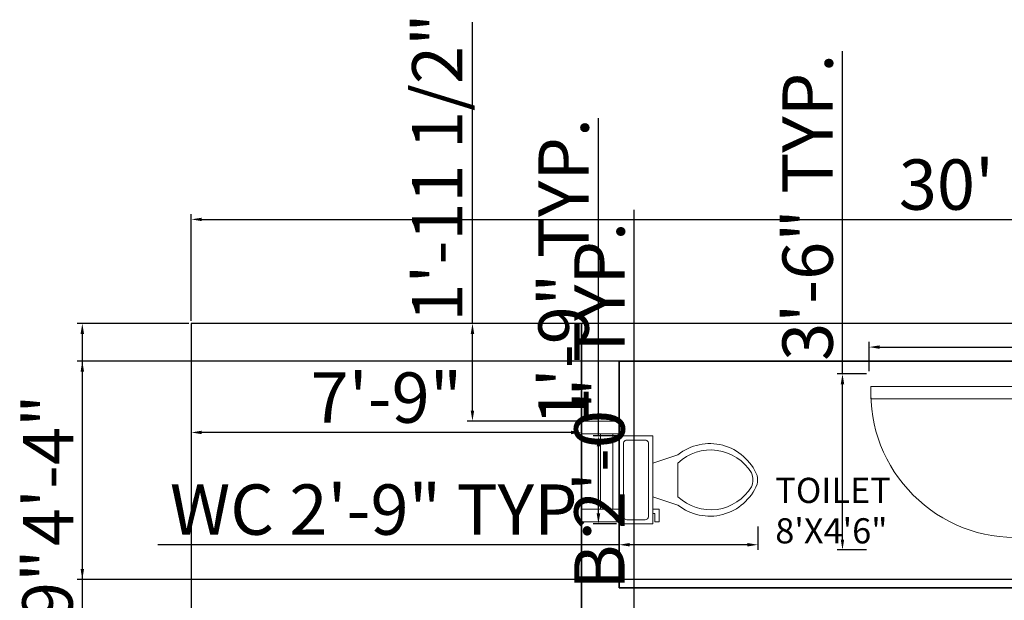
# Model space of a CAD drawing. Units: inches. Extents: x 2021 to 2692, y 429 to 1061.
# Tile 3 of 5: x 2127 to 2362, y 921 to 1059. Entities that reach past the tile are written whole.
import ezdxf

# ---------------------------------------------------------------- set-up
doc = ezdxf.new("R2010")
doc.units = ezdxf.units.IN
for name, color, linetype, lineweight in [('A-ANNO-DIMS', 2, 'Continuous', 18), ('A-AREA-IDEN', 7, 'Continuous', 18), ('A-DOOR', 4, 'Continuous', 18), ('A-FLOR-FIXT', 9, 'Continuous', 18), ('A-GLAZ', 4, 'Continuous', 18), ('A-WALL', 7, 'Continuous', 35), ('C-PROP', 3, 'Continuous', 25)]:
    doc.layers.add(name, color=color, linetype=linetype, lineweight=lineweight)
doc.styles.get("Standard").update_dxf_attribs({"font": 'arial.ttf'})
doc.dimstyles.new('ISO-25', dxfattribs={"dimtxt": 12, "dimasz": 2.5, "dimexe": 1.25, "dimexo": 0.625, "dimtad": 1, "dimdec": 0, "dimlunit": 3, "dimtxsty": 'Standard', "dimcen": 2.5, "dimadec": 0, "dimazin": 0, "dimtfac": 1, "dimtdec": 0, "dimtmove": 0, "dimatfit": 3, "dimfxl": 1, "dimarcsym": 0})

# ---------------------------------------------------------------- blocks, each defined once
blk = doc.blocks.new('Toilet - top')
for p, q in [((9.5, -6), (9.5, -2)), ((-10, -8.5), (-8, -8.5)), ((-10, -9.5), (-10, -8.5)), ((-8, -8.5), (-8, -8)), ((-7, -8), (-7, -9.5)), ((-4, -8), (-6, -14)), ((4, -8), (6, -14)), ((-7, -9.5), (-10, -9.5)), ((4, -14), (-4, -14))]:
    blk.add_line(p, q)
blk.add_lwpolyline([(10.5, -8), (10.5, 0), (-10.5, 0), (-10.5, -8)], close=True)
for points in [[(-9.5, -2), (-9.5, -6)], [(8.5, -1), (-8.5, -1)], [(-8.5, -7), (8.5, -7)]]:
    blk.add_lwpolyline(points)
for centre, radius, start, end in [((-8.62, -1.88), 0.884, 81.8699, 188.1301), ((8.62, -1.88), 0.884, 351.8699, 98.1301), ((-8.62, -6.12), 0.884, 171.8699, 278.1301), ((8.62, -6.12), 0.884, 261.8699, 8.1301), ((3.52, -21.58), 12.17, 141.4691, 247.9714), ((4.2, -21.82), 11.33, 136.3677, 238.9468), ((-3.52, -21.58), 12.17, 292.0284, 38.5307), ((-4.2, -21.82), 11.33, 301.053, 43.6321), ((0, -27.88), 4, 245.7318, 294.2682), ((0, -29), 4, 254.8605, 285.1395)]:
    blk.add_arc(centre, radius, start, end)
blk = doc.blocks.new('*D15')
at = {"layer": 'A-ANNO-DIMS', "color": 0, "lineweight": -2, "transparency": 16777216}
for p, q in [((2168.11, 987.59), (2168.11, 1013.02)), ((2170.61, 1011.77), (2525.61, 1011.77)), ((2528.11, 987.59), (2528.11, 1013.02))]:
    blk.add_line(p, q, dxfattribs=at)
at = {"layer": 'A-ANNO-DIMS', "color": 0, "transparency": 16777216}
for points in [[(2170.61, 1012.18), (2170.61, 1011.35), (2168.11, 1011.77)], [(2525.61, 1012.18), (2525.61, 1011.35), (2528.11, 1011.77)]]:
    blk.add_solid(points, dxfattribs=at)
at = {"layer": 'Defpoints', "color": 0, "transparency": 16777216}
for p in [(2528.11, 1011.77), (2168.11, 986.96), (2528.11, 986.96)]:
    blk.add_point(p, dxfattribs=at)
at = {"layer": 'A-ANNO-DIMS', "color": 0, "transparency": 16777216, "insert": (2348.11, 1018.52), "char_height": 12, "attachment_point": 5}
blk.add_mtext("30'", dxfattribs=at)
blk = doc.blocks.new('DOOR-SWING-36IN')
for p, q in [((36.03, 42), (42.03, 42)), ((36.03, 39), (42.03, 39)), ((36.03, 3), (42.03, 3)), ((36.03, 0), (42.03, 0))]:
    blk.add_line(p, q)
blk.add_lwpolyline([(36.03, 39), (0.03, 39), (0.03, 36), (36.03, 36)], close=True)
blk.add_arc((34.53, 37.5), 34.53, 177.5104, 272.4896)
blk = doc.blocks.new('WIN-18IN')
for p, q in [((9, 24), (0, 24)), ((0, 21), (0, 3)), ((9, 21), (0, 21)), ((4.5, 21), (4.5, 3)), ((7.5, 21), (7.5, 3)), ((9, 3), (9, 21)), ((0, 3), (9, 3)), ((0, 0), (9, 0))]:
    blk.add_line(p, q)
blk = doc.blocks.new('*D20')
at = {"layer": 'A-ANNO-DIMS', "color": 0, "lineweight": -2, "transparency": 16777216}
for p, q in [((2329.69, 975.59), (2329.69, 982.58)), ((2332.19, 981.33), (2369.61, 981.33)), ((2372.11, 975.59), (2372.11, 982.58)), ((2372.11, 981.33), (2531.32, 981.33))]:
    blk.add_line(p, q, dxfattribs=at)
at = {"layer": 'A-ANNO-DIMS', "color": 0, "transparency": 16777216}
for points in [[(2332.19, 981.74), (2332.19, 980.91), (2329.69, 981.33)], [(2369.61, 981.74), (2369.61, 980.91), (2372.11, 981.33)]]:
    blk.add_solid(points, dxfattribs=at)
at = {"layer": 'Defpoints', "color": 0, "transparency": 16777216}
for p in [(2372.11, 981.33), (2329.69, 974.96), (2372.11, 974.96)]:
    blk.add_point(p, dxfattribs=at)
at = {"layer": 'A-ANNO-DIMS', "color": 0, "transparency": 16777216, "insert": (2452.96, 988.17), "char_height": 12, "attachment_point": 5}
blk.add_mtext('DOOR 3\'-6 1/2" TYP.', dxfattribs=at)
blk = doc.blocks.new('*D21')
at = {"layer": 'A-ANNO-DIMS', "color": 0, "lineweight": -2, "transparency": 16777216}
for p, q in [((2323.33, 974.96), (2323.33, 1051.85)), ((2329.06, 974.96), (2322.08, 974.96)), ((2323.33, 935.46), (2323.33, 972.46)), ((2329.06, 932.96), (2322.08, 932.96))]:
    blk.add_line(p, q, dxfattribs=at)
at = {"layer": 'A-ANNO-DIMS', "color": 0, "transparency": 16777216}
for points in [[(2322.91, 972.46), (2323.74, 972.46), (2323.33, 974.96)], [(2322.91, 935.46), (2323.74, 935.46), (2323.33, 932.96)]]:
    blk.add_solid(points, dxfattribs=at)
at = {"layer": 'Defpoints', "color": 0, "transparency": 16777216}
for p in [(2323.33, 974.96), (2329.69, 974.96), (2329.69, 932.96)]:
    blk.add_point(p, dxfattribs=at)
at = {"layer": 'A-ANNO-DIMS', "color": 0, "transparency": 16777216, "insert": (2316.57, 1014.66), "char_height": 12, "attachment_point": 5, "rotation": 90}
blk.add_mtext('3\'-6" TYP.', dxfattribs=at)
blk = doc.blocks.new('*D34')
at = {"layer": 'A-ANNO-DIMS', "color": 0, "lineweight": -2, "transparency": 16777216}
for p, q in [((2270.11, 938.55), (2270.11, 932.96)), ((2303.16, 938.55), (2303.16, 932.96)), ((2270.11, 934.21), (2160.14, 934.21)), ((2300.66, 934.21), (2272.61, 934.21))]:
    blk.add_line(p, q, dxfattribs=at)
at = {"layer": 'A-ANNO-DIMS', "color": 0, "transparency": 16777216}
for points in [[(2272.61, 934.63), (2272.61, 933.8), (2270.11, 934.21)], [(2300.66, 934.63), (2300.66, 933.8), (2303.16, 934.21)]]:
    blk.add_solid(points, dxfattribs=at)
at = {"layer": 'Defpoints', "color": 0, "transparency": 16777216}
for p in [(2270.11, 939.17), (2303.16, 939.17), (2270.11, 934.21)]:
    blk.add_point(p, dxfattribs=at)
at = {"layer": 'A-ANNO-DIMS', "color": 0, "transparency": 16777216, "insert": (2213.87, 941.04), "char_height": 12, "attachment_point": 5}
blk.add_mtext('WC 2\'-9" TYP.', dxfattribs=at)
blk = doc.blocks.new('*D35')
at = {"layer": 'A-ANNO-DIMS', "color": 0, "lineweight": -2, "transparency": 16777216}
for p, q in [((2265.15, 960.17), (2265.15, 1035.94)), ((2269.48, 960.17), (2263.9, 960.17)), ((2265.15, 941.67), (2265.15, 957.67)), ((2269.48, 939.17), (2263.9, 939.17))]:
    blk.add_line(p, q, dxfattribs=at)
at = {"layer": 'A-ANNO-DIMS', "color": 0, "transparency": 16777216}
for points in [[(2264.74, 957.67), (2265.57, 957.67), (2265.15, 960.17)], [(2264.74, 941.67), (2265.57, 941.67), (2265.15, 939.17)]]:
    blk.add_solid(points, dxfattribs=at)
at = {"layer": 'Defpoints', "color": 0, "transparency": 16777216}
for p in [(2265.15, 960.17), (2270.11, 960.17), (2270.11, 939.17)]:
    blk.add_point(p, dxfattribs=at)
at = {"layer": 'A-ANNO-DIMS', "color": 0, "transparency": 16777216, "insert": (2258.4, 999.3), "char_height": 12, "attachment_point": 5, "rotation": 90}
blk.add_mtext('1\'-9" TYP.', dxfattribs=at)
blk = doc.blocks.new('*D36')
at = {"layer": 'A-ANNO-DIMS', "color": 0, "lineweight": -2, "transparency": 16777216}
for p, q in [((2273.71, 878.91), (2273.71, 1014.03)), ((2270.73, 878.91), (2274.96, 878.91)), ((2273.71, 857.41), (2273.71, 876.41)), ((2270.73, 854.91), (2274.96, 854.91))]:
    blk.add_line(p, q, dxfattribs=at)
at = {"layer": 'A-ANNO-DIMS', "color": 0, "transparency": 16777216}
for points in [[(2273.29, 876.41), (2274.13, 876.41), (2273.71, 878.91)], [(2273.29, 857.41), (2274.13, 857.41), (2273.71, 854.91)]]:
    blk.add_solid(points, dxfattribs=at)
at = {"layer": 'Defpoints', "color": 0, "transparency": 16777216}
for p in [(2270.11, 878.91), (2273.71, 878.91), (2270.11, 854.91)]:
    blk.add_point(p, dxfattribs=at)
at = {"layer": 'A-ANNO-DIMS', "color": 0, "transparency": 16777216, "insert": (2266.96, 947.72), "char_height": 12, "attachment_point": 5, "rotation": 90}
blk.add_mtext('WIN. B 2\'-0" TYP.', dxfattribs=at)
blk = doc.blocks.new('*D52')
at = {"layer": 'A-ANNO-DIMS', "color": 0, "lineweight": -2, "transparency": 16777216}
for p, q in [((2168.11, 986.34), (2168.11, 959.73)), ((2261.11, 986.34), (2261.11, 959.73)), ((2258.61, 960.98), (2170.61, 960.98))]:
    blk.add_line(p, q, dxfattribs=at)
at = {"layer": 'A-ANNO-DIMS', "color": 0, "transparency": 16777216}
for points in [[(2170.61, 961.4), (2170.61, 960.56), (2168.11, 960.98)], [(2258.61, 961.4), (2258.61, 960.56), (2261.11, 960.98)]]:
    blk.add_solid(points, dxfattribs=at)
at = {"layer": 'Defpoints', "color": 0, "transparency": 16777216}
for p in [(2168.11, 986.96), (2261.11, 986.96), (2168.11, 960.98)]:
    blk.add_point(p, dxfattribs=at)
at = {"layer": 'A-ANNO-DIMS', "color": 0, "transparency": 16777216, "insert": (2214.61, 967.73), "char_height": 12, "attachment_point": 5}
blk.add_mtext('7\'-9"', dxfattribs=at)
blk = doc.blocks.new('*D53')
at = {"layer": 'A-ANNO-DIMS', "color": 0, "lineweight": -2, "transparency": 16777216}
for p, q in [((2167.48, 986.96), (2140.87, 986.96)), ((2142.12, 984.46), (2142.12, 836.46)), ((2167.48, 833.96), (2140.87, 833.96))]:
    blk.add_line(p, q, dxfattribs=at)
at = {"layer": 'A-ANNO-DIMS', "color": 0, "transparency": 16777216}
for points in [[(2141.71, 984.46), (2142.54, 984.46), (2142.12, 986.96)], [(2141.71, 836.46), (2142.54, 836.46), (2142.12, 833.96)]]:
    blk.add_solid(points, dxfattribs=at)
at = {"layer": 'Defpoints', "color": 0, "transparency": 16777216}
for p in [(2168.11, 986.96), (2142.12, 833.96), (2168.11, 833.96)]:
    blk.add_point(p, dxfattribs=at)
at = {"layer": 'A-ANNO-DIMS', "color": 0, "transparency": 16777216, "insert": (2135.37, 910.46), "char_height": 12, "attachment_point": 5, "rotation": 90}
blk.add_mtext('12\'-9"', dxfattribs=at)
blk = doc.blocks.new('*D63')
at = {"layer": 'A-ANNO-DIMS', "color": 0, "lineweight": -2, "transparency": 16777216}
for p, q in [((2518.48, 977.96), (2140.87, 977.96)), ((2142.12, 975.46), (2142.12, 928.44)), ((2518.48, 925.94), (2140.87, 925.94))]:
    blk.add_line(p, q, dxfattribs=at)
at = {"layer": 'A-ANNO-DIMS', "color": 0, "transparency": 16777216}
for points in [[(2141.71, 975.46), (2142.54, 975.46), (2142.12, 977.96)], [(2141.71, 928.44), (2142.54, 928.44), (2142.12, 925.94)]]:
    blk.add_solid(points, dxfattribs=at)
at = {"layer": 'Defpoints', "color": 0, "transparency": 16777216}
for p in [(2519.11, 977.96), (2142.12, 925.94), (2519.11, 925.94)]:
    blk.add_point(p, dxfattribs=at)
at = {"layer": 'A-ANNO-DIMS', "color": 0, "transparency": 16777216, "insert": (2135.5, 951.95), "char_height": 12, "attachment_point": 5, "rotation": 90}
blk.add_mtext('4\'-4"', dxfattribs=at)
blk = doc.blocks.new('*D66')
at = {"layer": 'A-ANNO-DIMS', "color": 0, "lineweight": -2, "transparency": 16777216}
for p, q in [((2235.12, 986.96), (2235.12, 1058.77)), ((2260.48, 986.96), (2233.87, 986.96)), ((2235.12, 966.19), (2235.12, 984.46)), ((2260.48, 963.69), (2233.87, 963.69))]:
    blk.add_line(p, q, dxfattribs=at)
at = {"layer": 'A-ANNO-DIMS', "color": 0, "transparency": 16777216}
for points in [[(2234.71, 984.46), (2235.54, 984.46), (2235.12, 986.96)], [(2234.71, 966.19), (2235.54, 966.19), (2235.12, 963.69)]]:
    blk.add_solid(points, dxfattribs=at)
at = {"layer": 'Defpoints', "color": 0, "transparency": 16777216}
for p in [(2235.12, 986.96), (2261.11, 986.96), (2261.11, 963.69)]:
    blk.add_point(p, dxfattribs=at)
at = {"layer": 'A-ANNO-DIMS', "color": 0, "transparency": 16777216, "insert": (2228.3, 1024.12), "char_height": 12, "attachment_point": 5, "rotation": 90}
blk.add_mtext('1\'-11 1/2"', dxfattribs=at)

msp = doc.modelspace()

# ---------------------------------------------------------------- linework, layer by layer
at = {"layer": 'A-WALL'}
for p, q in [((2261.11, 923.96), (2261.11, 986.96)), ((2366.11, 977.96), (2270.11, 977.96)), ((2270.11, 923.96), (2270.11, 977.96)), ((2261.11, 833.96), (2261.11, 939.69)), ((2366.11, 923.96), (2270.11, 923.96))]:
    msp.add_line(p, q, dxfattribs=at)
at = {"layer": 'C-PROP'}
msp.add_lwpolyline([(2168.11, 506.96), (2528.11, 506.96), (2528.11, 986.96), (2168.11, 986.96)], close=True, dxfattribs=at)

# ---------------------------------------------------------------- block references
at = {"layer": 'A-DOOR'}
msp.add_blockref('DOOR-SWING-36IN', (2330.08, 932.96), dxfattribs=at)
at = {"layer": 'A-FLOR-FIXT', "rotation": 90}
msp.add_blockref('Toilet - top', (2270.11, 949.67), dxfattribs=at)
at = {"layer": 'A-GLAZ'}
msp.add_blockref('WIN-18IN', (2261.11, 939.69), dxfattribs=at)

# ---------------------------------------------------------------- texts
at = {"layer": 'A-AREA-IDEN'}
for s, p in [('TOILET', (2307.31, 944.17)), ('8\'X4\'6"', (2307.31, 934.53))]:
    msp.add_text(s, height=6, dxfattribs=at).set_placement(p)

# ---------------------------------------------------------------- dimensions: what is measured, and where the dimension line sits
at = {"layer": 'A-ANNO-DIMS'}
for base, p1, p2, angle, picture, middle in [((2235.12, 986.96), (2261.11, 963.69), (2261.11, 986.96), 90, '*D66', (2228.3, 1024.12)), ((2142.12, 833.96), (2168.11, 986.96), (2168.11, 833.96), 90, '*D53', (2135.37, 910.46)), ((2168.11, 960.98), (2261.11, 986.96), (2168.11, 986.96), 180, '*D52', (2214.61, 967.73)), ((2142.12, 925.94), (2519.11, 977.96), (2519.11, 925.94), 90, '*D63', (2135.5, 951.95))]:
    dim = msp.add_linear_dim(base=base, p1=p1, p2=p2, angle=angle, dimstyle='ISO-25', override={"dimdec": 1, "dimlfac": 1, "dimrnd": 0, "dimzin": 1, "dimdsep": 46, "dimlunit": 4, "dimfrac": 2}, dxfattribs=at)
    dim.commit()
    dim.dimension.update_dxf_attribs({"geometry": picture, "text_midpoint": middle})
for base, p1, p2, angle, text, picture, middle in [((2323.33, 974.96), (2329.69, 932.96), (2329.69, 974.96), 90, '<> TYP.', '*D21', (2316.57, 1014.66)), ((2265.15, 960.17), (2270.11, 939.17), (2270.11, 960.17), 90, '<> TYP.', '*D35', (2258.4, 999.3)), ((2273.71, 878.91), (2270.11, 854.91), (2270.11, 878.91), 90, 'WIN. B <> TYP.', '*D36', (2266.96, 947.72)), ((2270.1097, 934.2138), (2303.156, 939.1708), (2270.1097, 939.1708), 180, 'WC <> TYP.', '*D34', (2213.8729, 941.0435))]:
    dim = msp.add_linear_dim(base=base, p1=p1, p2=p2, angle=angle, text=text, dimstyle='ISO-25', override={"dimdec": 1, "dimlfac": 1, "dimrnd": 0, "dimzin": 1, "dimdsep": 46, "dimlunit": 4, "dimfrac": 2}, dxfattribs=at)
    dim.commit()
    dim.dimension.update_dxf_attribs({"geometry": picture, "text_midpoint": middle})
dim = msp.add_linear_dim(base=(2528.11, 1011.77), p1=(2168.11, 986.96), p2=(2528.11, 986.96), dimstyle='ISO-25', override={"dimclrd": 0, "dimclre": 0, "dimclrt": 0}, dxfattribs=at)
dim.commit()
dim.dimension.update_dxf_attribs({"geometry": '*D15', "text_midpoint": (2348.11, 1018.52)})
dim = msp.add_linear_dim(base=(2372.11, 981.33), p1=(2329.69, 974.96), p2=(2372.11, 974.96), text='DOOR <> TYP.', dimstyle='ISO-25', override={"dimdec": 1, "dimlfac": 1, "dimrnd": 0, "dimzin": 1, "dimdsep": 46, "dimlunit": 4, "dimfrac": 2}, dxfattribs=at)
dim.commit()
dim.dimension.update_dxf_attribs({"geometry": '*D20', "text_midpoint": (2452.96, 988.17)})

doc.saveas('drawing.dxf')
